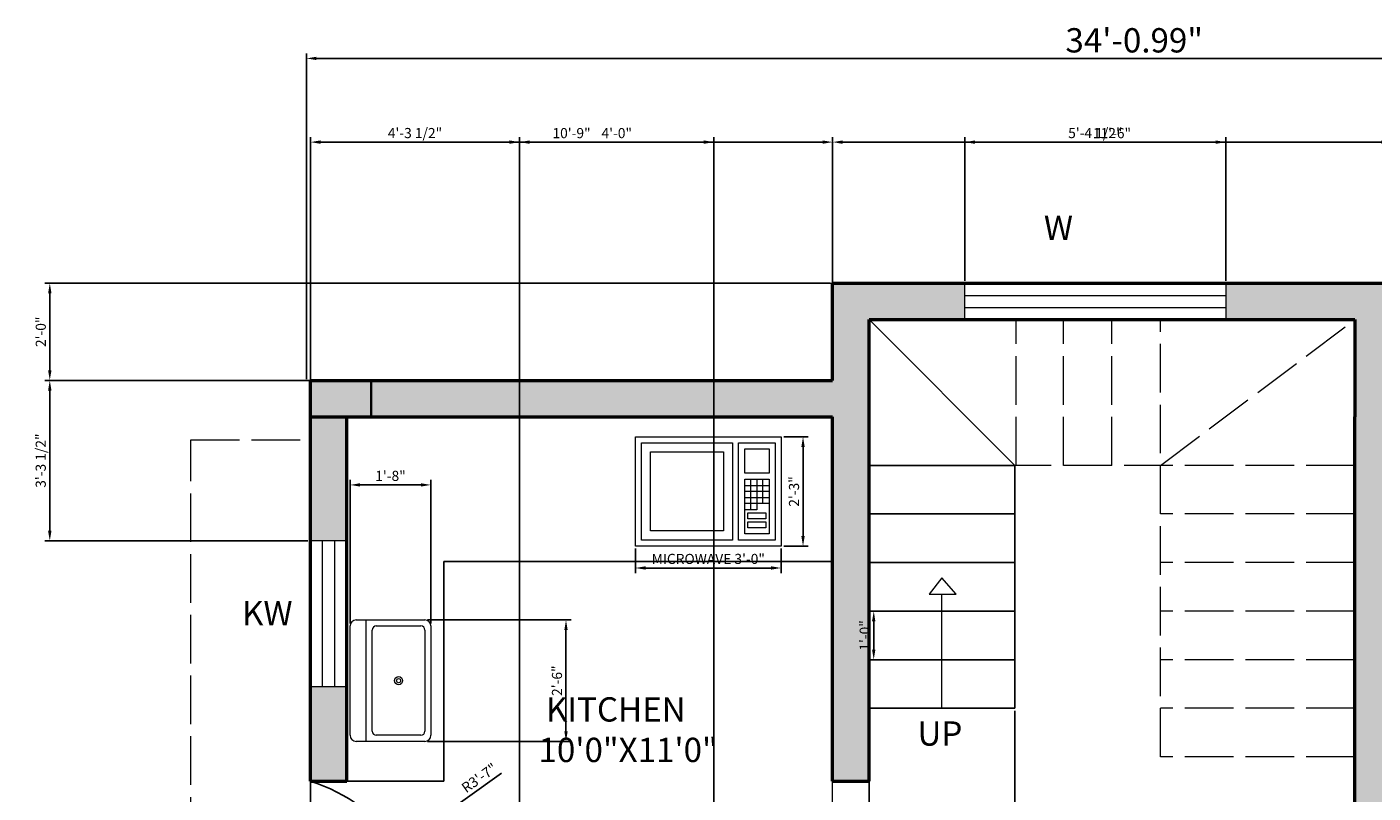
# Model space of a CAD drawing. Units: inches. Extents: x 5703 to 6226, y 10088 to 10813.
# Tile 4 of 5: x 5703 to 6036, y 10624 to 10813. Entities that reach past the tile are written whole.
import ezdxf

# ---------------------------------------------------------------- set-up
doc = ezdxf.new("R2010")
doc.units = ezdxf.units.IN
doc.linetypes.add('ACAD_ISO02W100', pattern=[15, 12, -3])
for name, color, linetype, lineweight in [('A-ANNO-DIMS', 2, 'Continuous', 18), ('A-ANNO-SYMB', 7, 'Continuous', 18), ('A-ANNO-TEXT', 7, 'Continuous', 18), ('A-AREA-IDEN', 7, 'Continuous', 18), ('A-COLS', 7, 'Continuous', 35), ('A-COLS-PATT', 7, 'Continuous', 13), ('A-DOOR', 140, 'Continuous', 25), ('A-EQPM', 8, 'Continuous', 18), ('A-FLOR-CASE', 8, 'Continuous', 25), ('A-FLOR-FIXT', 8, 'Continuous', 18), ('A-FLOR-STRS', 7, 'Continuous', 25), ('A-WALL', 7, 'Continuous', 50), ('A-WALL-PATT', 9, 'Continuous', 13)]:
    doc.layers.add(name, color=color, linetype=linetype, lineweight=lineweight)
for name, color, linetype, lineweight, true_color in [('A-FLOR-STRS-OVHD', 217, 'ACAD_ISO02W100', 18, 0x93278f), ('A-GLAZ', 112, 'Continuous', 18, 0x1ce368), ('A-ROOF-OVHD', 30, 'ACAD_ISO02W100', 18, 0xf8991e), ('A-WALL-OVHD', 30, 'ACAD_ISO02W100', 18, 0xf8991e)]:
    doc.layers.add(name, color=color, linetype=linetype, lineweight=lineweight, true_color=true_color)
doc.styles.get("Standard").update_dxf_attribs({"font": 'arial.ttf'})
doc.dimstyles.new('ISO-25', dxfattribs={"dimtxt": 2.5, "dimasz": 2.5, "dimexe": 1.25, "dimexo": 0.625, "dimtad": 1, "dimlunit": 3, "dimtxsty": 'Standard', "dimcen": 2.5, "dimadec": 0, "dimazin": 0, "dimtfac": 1, "dimtmove": 0, "dimatfit": 3, "dimfxl": 1, "dimarcsym": 0})

# ---------------------------------------------------------------- blocks, each defined once
blk = doc.blocks.new('*D10')
at = {"layer": 'A-ANNO-DIMS', "color": 0, "lineweight": -2, "transparency": 16777216}
for p, q in [((5772.18, 10726.21), (5772.18, 10806.65)), ((5774.68, 10805.4), (6178.68, 10805.4)), ((6181.18, 10726.49), (6181.18, 10806.65))]:
    blk.add_line(p, q, dxfattribs=at)
at = {"layer": 'A-ANNO-DIMS', "color": 0, "transparency": 16777216}
for points in [[(5774.68, 10805.81), (5774.68, 10804.98), (5772.18, 10805.4)], [(6178.68, 10805.81), (6178.68, 10804.98), (6181.18, 10805.4)]]:
    blk.add_solid(points, dxfattribs=at)
at = {"layer": 'Defpoints', "color": 0, "transparency": 16777216}
for p in [(6181.18, 10805.4), (5772.18, 10725.59), (6181.18, 10725.87)]:
    blk.add_point(p, dxfattribs=at)
at = {"layer": 'A-ANNO-DIMS', "color": 0, "transparency": 16777216, "insert": (5976.68, 10809.09), "char_height": 6, "attachment_point": 5}
blk.add_mtext('34\'-0.99"', dxfattribs=at)
blk = doc.blocks.new('Microwave')
for p, q in [((18, 10), (22, 10)), ((22, 9), (18, 9)), ((19, 7), (19, 11)), ((20, 11), (20, 7)), ((21, 7), (21, 11)), ((18, 8), (22, 8)), ((22, 7), (18, 7)), ((19, 6), (19, 7)), ((20, 7), (20, 6)), ((20, 6), (18, 6))]:
    blk.add_line(p, q)
for points in [[(0, 0), (0, 18), (24, 18), (24, 0)], [(1, 1), (1, 17), (16, 17), (16, 1)], [(17, 1), (17, 17), (23, 17), (23, 1)], [(18, 12), (18, 16), (22, 16), (22, 12)], [(2.5, 2.5), (2.5, 15.5), (14.5, 15.5), (14.5, 2.5)], [(18, 2), (18, 11), (22, 11), (22, 2)], [(18.5, 4.5), (18.5, 5.5), (21.5, 5.5), (21.5, 4.5)], [(18.5, 3), (18.5, 4), (21.5, 4), (21.5, 3)]]:
    blk.add_lwpolyline(points, close=True)
blk = doc.blocks.new('Sink-single - 30 in top')
blk.add_line((-15, -3.999996), (15, -3.999996))
for points in [[(-13.5, 0), (13.5, 0)], [(-15, -18.499996), (-15, -1.5)], [(15, -1.5), (15, -18.499996)], [(-13.5, -17.499996), (-13.5, -6.499996)], [(-12.5, -5.499996), (12.5, -5.499996)], [(13.5, -6.499996), (13.5, -17.499996)], [(12.5, -18.499996), (-12.5, -18.499996)], [(13.5, -19.999996), (-13.5, -19.999996)]]:
    blk.add_lwpolyline(points)
for radius in [1, 0.5]:
    blk.add_circle((0, -11.999996), radius)
for centre, radius, start, end in [((-13.5, -1.5), 1.5, 90, 180), ((13.5, -1.5), 1.5, 0, 90), ((-12.5, -6.499996), 1, 90, 180), ((12.5, -6.499996), 1, 0, 90), ((-13.5, -18.499996), 1.5, 180, 270), ((-12.5, -17.499996), 1, 180, 270), ((12.5, -17.499996), 1, 270, 0), ((13.5, -18.499996), 1.5, 270, 0)]:
    blk.add_arc(centre, radius, start, end)
blk = doc.blocks.new('WIN-36x9')
for p, q in [((0, 9), (0, 0)), ((36, 9), (0, 9)), ((36, 0), (36, 9)), ((36, 6), (0, 6)), ((36, 3), (0, 3)), ((0, 0), (36, 0))]:
    blk.add_line(p, q)
blk = doc.blocks.new('*D28')
at = {"layer": 'A-ANNO-DIMS', "color": 0, "lineweight": -2, "transparency": 16777216}
for p, q in [((5853.46, 10684.31), (5853.46, 10678.28)), ((5889.46, 10684.31), (5889.46, 10678.28)), ((5855.96, 10679.53), (5886.96, 10679.53))]:
    blk.add_line(p, q, dxfattribs=at)
at = {"layer": 'A-ANNO-DIMS', "color": 0, "transparency": 16777216}
for points in [[(5855.96, 10679.95), (5855.96, 10679.12), (5853.46, 10679.53)], [(5886.96, 10679.95), (5886.96, 10679.12), (5889.46, 10679.53)]]:
    blk.add_solid(points, dxfattribs=at)
at = {"layer": 'Defpoints', "color": 0, "transparency": 16777216}
for p in [(5853.46, 10684.93), (5889.46, 10684.93), (5889.46, 10679.53)]:
    blk.add_point(p, dxfattribs=at)
at = {"layer": 'A-ANNO-DIMS', "color": 0, "transparency": 16777216, "insert": (5871.46, 10681.45), "char_height": 2.5, "attachment_point": 5}
blk.add_mtext('MICROWAVE 3\'-0"', dxfattribs=at)
blk = doc.blocks.new('*D29')
at = {"layer": 'A-ANNO-DIMS', "color": 0, "lineweight": -2, "transparency": 16777216}
for p, q in [((5890.09, 10711.93), (5896.11, 10711.93)), ((5894.86, 10687.43), (5894.86, 10709.43)), ((5890.09, 10684.93), (5896.11, 10684.93))]:
    blk.add_line(p, q, dxfattribs=at)
at = {"layer": 'A-ANNO-DIMS', "color": 0, "transparency": 16777216}
for points in [[(5894.45, 10709.43), (5895.28, 10709.43), (5894.86, 10711.93)], [(5894.45, 10687.43), (5895.28, 10687.43), (5894.86, 10684.93)]]:
    blk.add_solid(points, dxfattribs=at)
at = {"layer": 'Defpoints', "color": 0, "transparency": 16777216}
for p in [(5889.46, 10711.93), (5894.86, 10711.93), (5889.46, 10684.93)]:
    blk.add_point(p, dxfattribs=at)
at = {"layer": 'A-ANNO-DIMS', "color": 0, "transparency": 16777216, "insert": (5892.96, 10698.43), "char_height": 2.5, "attachment_point": 5, "rotation": 90}
blk.add_mtext('2\'-3"', dxfattribs=at)
blk = doc.blocks.new('*D36')
at = {"layer": 'A-ANNO-DIMS', "color": 0, "lineweight": -2, "transparency": 16777216}
for p, q in [((5782.96, 10665.83), (5782.96, 10701.3)), ((5802.96, 10665.83), (5802.96, 10701.3)), ((5785.46, 10700.05), (5800.46, 10700.05))]:
    blk.add_line(p, q, dxfattribs=at)
at = {"layer": 'A-ANNO-DIMS', "color": 0, "transparency": 16777216}
for points in [[(5785.46, 10700.47), (5785.46, 10699.64), (5782.96, 10700.05)], [(5800.46, 10700.47), (5800.46, 10699.64), (5802.96, 10700.05)]]:
    blk.add_solid(points, dxfattribs=at)
at = {"layer": 'Defpoints', "color": 0, "transparency": 16777216}
for p in [(5802.96, 10700.05), (5782.96, 10665.2), (5802.96, 10665.2)]:
    blk.add_point(p, dxfattribs=at)
at = {"layer": 'A-ANNO-DIMS', "color": 0, "transparency": 16777216, "insert": (5792.96, 10701.96), "char_height": 2.5, "attachment_point": 5}
blk.add_mtext('1\'-8"', dxfattribs=at)
blk = doc.blocks.new('*D37')
at = {"layer": 'A-ANNO-DIMS', "color": 0, "lineweight": -2, "transparency": 16777216}
for p, q in [((5802.09, 10666.7), (5837.56, 10666.7)), ((5836.31, 10664.2), (5836.31, 10639.2)), ((5802.09, 10636.7), (5837.56, 10636.7))]:
    blk.add_line(p, q, dxfattribs=at)
at = {"layer": 'A-ANNO-DIMS', "color": 0, "transparency": 16777216}
for points in [[(5835.9, 10664.2), (5836.73, 10664.2), (5836.31, 10666.7)], [(5835.9, 10639.2), (5836.73, 10639.2), (5836.31, 10636.7)]]:
    blk.add_solid(points, dxfattribs=at)
at = {"layer": 'Defpoints', "color": 0, "transparency": 16777216}
for p in [(5801.46, 10666.7), (5801.46, 10636.7), (5836.31, 10636.7)]:
    blk.add_point(p, dxfattribs=at)
at = {"layer": 'A-ANNO-DIMS', "color": 0, "transparency": 16777216, "insert": (5834.41, 10651.7), "char_height": 2.5, "attachment_point": 5, "rotation": 90}
blk.add_mtext('2\'-6"', dxfattribs=at)
blk = doc.blocks.new('*D40')
at = {"layer": 'A-ANNO-DIMS', "color": 0, "lineweight": -2, "transparency": 16777216}
for p, q in [((5911.18, 10644.24), (5911.18, 10088.29)), ((5947.18, 10644.24), (5947.18, 10088.29)), ((5913.68, 10089.54), (5944.68, 10089.54))]:
    blk.add_line(p, q, dxfattribs=at)
at = {"layer": 'A-ANNO-DIMS', "color": 0, "transparency": 16777216}
for points in [[(5913.68, 10089.96), (5913.68, 10089.12), (5911.18, 10089.54)], [(5944.68, 10089.96), (5944.68, 10089.12), (5947.18, 10089.54)]]:
    blk.add_solid(points, dxfattribs=at)
at = {"layer": 'Defpoints', "color": 0, "transparency": 16777216}
for p in [(5911.18, 10644.87), (5947.18, 10644.87), (5947.18, 10089.54)]:
    blk.add_point(p, dxfattribs=at)
at = {"layer": 'A-ANNO-DIMS', "color": 0, "transparency": 16777216, "insert": (5929.18, 10091.44), "char_height": 2.5, "attachment_point": 5}
blk.add_mtext('3\'-0"', dxfattribs=at)
blk = doc.blocks.new('*D41')
at = {"layer": 'A-ANNO-DIMS', "color": 0, "lineweight": -2, "transparency": 16777216}
for p, q in [((5946.55, 10668.87), (5911.08, 10668.87)), ((5912.33, 10659.37), (5912.33, 10666.37)), ((5946.55, 10656.87), (5911.08, 10656.87))]:
    blk.add_line(p, q, dxfattribs=at)
at = {"layer": 'A-ANNO-DIMS', "color": 0, "transparency": 16777216}
for points in [[(5911.91, 10666.37), (5912.74, 10666.37), (5912.33, 10668.87)], [(5911.91, 10659.37), (5912.74, 10659.37), (5912.33, 10656.87)]]:
    blk.add_solid(points, dxfattribs=at)
at = {"layer": 'Defpoints', "color": 0, "transparency": 16777216}
for p in [(5912.33, 10668.87), (5947.18, 10668.87), (5947.18, 10656.87)]:
    blk.add_point(p, dxfattribs=at)
at = {"layer": 'A-ANNO-DIMS', "color": 0, "transparency": 16777216, "insert": (5910.42, 10662.87), "char_height": 2.5, "attachment_point": 5, "rotation": 90}
blk.add_mtext('1\'-0"', dxfattribs=at)
blk = doc.blocks.new('*D43')
at = {"layer": 'A-ANNO-DIMS', "color": 0, "lineweight": -2, "transparency": 16777216}
for p, q in [((5773.18, 10726.49), (5773.18, 10785.97)), ((5775.68, 10784.72), (5899.68, 10784.72)), ((5902.18, 10726.49), (5902.18, 10785.97))]:
    blk.add_line(p, q, dxfattribs=at)
at = {"layer": 'A-ANNO-DIMS', "color": 0, "transparency": 16777216}
for points in [[(5775.68, 10785.14), (5775.68, 10784.3), (5773.18, 10784.72)], [(5899.68, 10785.14), (5899.68, 10784.3), (5902.18, 10784.72)]]:
    blk.add_solid(points, dxfattribs=at)
at = {"layer": 'Defpoints', "color": 0, "transparency": 16777216}
for p in [(5902.18, 10784.72), (5773.18, 10725.87), (5902.18, 10725.87)]:
    blk.add_point(p, dxfattribs=at)
at = {"layer": 'A-ANNO-DIMS', "color": 0, "transparency": 16777216, "insert": (5837.68, 10786.62), "char_height": 2.5, "attachment_point": 5}
blk.add_mtext('10\'-9"', dxfattribs=at)
blk = doc.blocks.new('*D44')
at = {"layer": 'A-ANNO-DIMS', "color": 0, "lineweight": -2, "transparency": 16777216}
for p, q in [((5902.18, 10750.49), (5902.18, 10785.97)), ((5904.68, 10784.72), (6037.68, 10784.72)), ((6040.18, 10750.49), (6040.18, 10785.97))]:
    blk.add_line(p, q, dxfattribs=at)
at = {"layer": 'A-ANNO-DIMS', "color": 0, "transparency": 16777216}
for points in [[(5904.68, 10785.14), (5904.68, 10784.3), (5902.18, 10784.72)], [(6037.68, 10785.14), (6037.68, 10784.3), (6040.18, 10784.72)]]:
    blk.add_solid(points, dxfattribs=at)
at = {"layer": 'Defpoints', "color": 0, "transparency": 16777216}
for p in [(6040.18, 10784.72), (5902.18, 10749.87), (6040.18, 10749.87)]:
    blk.add_point(p, dxfattribs=at)
at = {"layer": 'A-ANNO-DIMS', "color": 0, "transparency": 16777216, "insert": (5971.18, 10786.62), "char_height": 2.5, "attachment_point": 5}
blk.add_mtext('11\'-6"', dxfattribs=at)
blk = doc.blocks.new('*D45')
at = {"layer": 'A-ANNO-DIMS', "color": 0, "lineweight": -2, "transparency": 16777216}
for p, q in [((5901.55, 10749.87), (5707.55, 10749.87)), ((5708.8, 10728.37), (5708.8, 10747.37)), ((5901.55, 10725.87), (5707.55, 10725.87))]:
    blk.add_line(p, q, dxfattribs=at)
at = {"layer": 'A-ANNO-DIMS', "color": 0, "transparency": 16777216}
for points in [[(5708.38, 10747.37), (5709.22, 10747.37), (5708.8, 10749.87)], [(5708.38, 10728.37), (5709.22, 10728.37), (5708.8, 10725.87)]]:
    blk.add_solid(points, dxfattribs=at)
at = {"layer": 'Defpoints', "color": 0, "transparency": 16777216}
for p in [(5708.8, 10749.87), (5902.18, 10749.87), (5902.18, 10725.87)]:
    blk.add_point(p, dxfattribs=at)
at = {"layer": 'A-ANNO-DIMS', "color": 0, "transparency": 16777216, "insert": (5706.9, 10737.87), "char_height": 2.5, "attachment_point": 5, "rotation": 90}
blk.add_mtext('2\'-0"', dxfattribs=at)
blk = doc.blocks.new('*D46')
at = {"layer": 'A-ANNO-DIMS', "color": 0, "lineweight": -2, "transparency": 16777216}
for p, q in [((5934.86, 10750.49), (5934.86, 10785.97)), ((5937.36, 10784.72), (5996.77, 10784.72)), ((5999.27, 10750.49), (5999.27, 10785.97))]:
    blk.add_line(p, q, dxfattribs=at)
at = {"layer": 'A-ANNO-DIMS', "color": 0, "transparency": 16777216}
for points in [[(5937.36, 10785.14), (5937.36, 10784.3), (5934.86, 10784.72)], [(5996.77, 10785.14), (5996.77, 10784.3), (5999.27, 10784.72)]]:
    blk.add_solid(points, dxfattribs=at)
at = {"layer": 'Defpoints', "color": 0, "transparency": 16777216}
for p in [(5999.27, 10784.72), (5934.86, 10749.87), (5999.27, 10749.87)]:
    blk.add_point(p, dxfattribs=at)
at = {"layer": 'A-ANNO-DIMS', "color": 0, "transparency": 16777216, "insert": (5967.07, 10786.64), "char_height": 2.5, "attachment_point": 5}
blk.add_mtext('5\'-4 1/2"', dxfattribs=at)
blk = doc.blocks.new('*D47')
at = {"layer": 'A-ANNO-DIMS', "color": 0, "lineweight": -2, "transparency": 16777216}
for p, q in [((5824.85, 10313.99), (5824.85, 10785.97)), ((5827.35, 10784.72), (5870.35, 10784.72)), ((5872.85, 10313.99), (5872.85, 10785.97))]:
    blk.add_line(p, q, dxfattribs=at)
at = {"layer": 'A-ANNO-DIMS', "color": 0, "transparency": 16777216}
for points in [[(5827.35, 10785.14), (5827.35, 10784.3), (5824.85, 10784.72)], [(5870.35, 10785.14), (5870.35, 10784.3), (5872.85, 10784.72)]]:
    blk.add_solid(points, dxfattribs=at)
at = {"layer": 'Defpoints', "color": 0, "transparency": 16777216}
for p in [(5872.85, 10784.72), (5824.85, 10313.37), (5872.85, 10313.37)]:
    blk.add_point(p, dxfattribs=at)
at = {"layer": 'A-ANNO-DIMS', "color": 0, "transparency": 16777216, "insert": (5848.85, 10786.62), "char_height": 2.5, "attachment_point": 5}
blk.add_mtext('4\'-0"', dxfattribs=at)
blk = doc.blocks.new('*D48')
at = {"layer": 'A-ANNO-DIMS', "color": 0, "lineweight": -2, "transparency": 16777216}
for p, q in [((5773.18, 10304.99), (5773.18, 10785.97)), ((5775.68, 10784.72), (5822.35, 10784.72)), ((5824.85, 10304.99), (5824.85, 10785.97))]:
    blk.add_line(p, q, dxfattribs=at)
at = {"layer": 'A-ANNO-DIMS', "color": 0, "transparency": 16777216}
for points in [[(5775.68, 10785.14), (5775.68, 10784.3), (5773.18, 10784.72)], [(5822.35, 10785.14), (5822.35, 10784.3), (5824.85, 10784.72)]]:
    blk.add_solid(points, dxfattribs=at)
at = {"layer": 'Defpoints', "color": 0, "transparency": 16777216}
for p in [(5824.85, 10784.72), (5773.18, 10304.37), (5824.85, 10304.37)]:
    blk.add_point(p, dxfattribs=at)
at = {"layer": 'A-ANNO-DIMS', "color": 0, "transparency": 16777216, "insert": (5799.01, 10786.64), "char_height": 2.5, "attachment_point": 5}
blk.add_mtext('4\'-3 1/2"', dxfattribs=at)
blk = doc.blocks.new('*D50')
at = {"layer": 'A-ANNO-DIMS', "color": 0, "lineweight": -2, "transparency": 16777216}
for p, q in [((5772.55, 10725.87), (5707.55, 10725.87)), ((5708.8, 10688.73), (5708.8, 10723.37)), ((5772.55, 10686.23), (5707.55, 10686.23))]:
    blk.add_line(p, q, dxfattribs=at)
at = {"layer": 'A-ANNO-DIMS', "color": 0, "transparency": 16777216}
for points in [[(5708.38, 10723.37), (5709.22, 10723.37), (5708.8, 10725.87)], [(5708.38, 10688.73), (5709.22, 10688.73), (5708.8, 10686.23)]]:
    blk.add_solid(points, dxfattribs=at)
at = {"layer": 'Defpoints', "color": 0, "transparency": 16777216}
for p in [(5708.8, 10725.87), (5773.18, 10725.87), (5773.18, 10686.23)]:
    blk.add_point(p, dxfattribs=at)
at = {"layer": 'A-ANNO-DIMS', "color": 0, "transparency": 16777216, "insert": (5706.88, 10706.05), "char_height": 2.5, "attachment_point": 5, "rotation": 90}
blk.add_mtext('3\'-3 1/2"', dxfattribs=at)
blk = doc.blocks.new('*D58')
at = {"layer": 'A-ANNO-DIMS', "color": 0, "lineweight": -2, "transparency": 16777216}
for p, q in [((5820.36, 10628.86), (5797.21, 10612.32)), ((5760.18, 10585.87), (5795.18, 10610.87))]:
    blk.add_line(p, q, dxfattribs=at)
at = {"layer": 'A-ANNO-DIMS', "color": 0, "transparency": 16777216}
blk.add_solid([(5796.97, 10612.66), (5797.45, 10611.98), (5795.18, 10610.87)], dxfattribs=at)
at = {"layer": 'Defpoints', "color": 0, "transparency": 16777216}
for p in [(5795.18, 10610.87), (5760.18, 10585.87)]:
    blk.add_point(p, dxfattribs=at)
at = {"layer": 'A-ANNO-DIMS', "color": 0, "transparency": 16777216, "insert": (5815.07, 10627.42), "char_height": 2.5, "attachment_point": 5, "rotation": 35.5383}
blk.add_mtext('R3\'-7"', dxfattribs=at)

msp = doc.modelspace()

# ---------------------------------------------------------------- hatches: boundary and pattern name
at = {"layer": 'A-COLS-PATT'}
h = msp.add_hatch(color=256, dxfattribs=at)
h.dxf.hatch_style = 1
h.paths.add_polyline_path([(5788.176, 10725.869), (5773.176, 10725.869), (5773.176, 10716.869), (5788.176, 10716.869)])
h.paths.add_polyline_path([(5782.176, 10516.684), (5773.176, 10516.684), (5773.176, 10497.849), (5782.176, 10497.849)])
h.paths.add_polyline_path([(5782.176, 10319.369), (5773.176, 10319.369), (5773.176, 10304.369), (5782.176, 10304.369)])
h.paths.add_polyline_path([(5960.955, 10313.369), (5953.525, 10313.369), (5953.525, 10304.369), (5960.955, 10304.369)])
h.paths.add_polyline_path([(6040.176, 10314.869), (6031.176, 10314.869), (6031.176, 10304.369), (6040.176, 10304.369)])
h.paths.add_polyline_path([(6181.176, 10198.545), (6172.176, 10198.545), (6172.176, 10178.369), (6181.176, 10178.369)])
h.paths.add_polyline_path([(6181.176, 10505.369), (6172.176, 10505.369), (6172.176, 10492.633), (6181.176, 10492.633)])
h.paths.add_polyline_path([(6181.176, 10725.869), (6166.176, 10725.869), (6166.176, 10716.869), (6181.176, 10716.869)])
at = {"layer": 'A-WALL-PATT'}
h = msp.add_hatch(color=256, dxfattribs=at)
h.dxf.hatch_style = 1
h.paths.add_polyline_path([(6057.982, 10725.869), (6040.176, 10725.869), (6040.176, 10749.869), (5999.271, 10749.869), (5999.271, 10740.869), (6031.176, 10740.869), (6031.176, 10716.869), (6031.176, 10511.369), (6013.525, 10511.369), (6013.525, 10505.369), (6048.161, 10505.369), (6048.161, 10511.369), (6040.176, 10511.369), (6040.176, 10716.869), (6057.982, 10716.869)])
h.paths.add_polyline_path([(6166.176, 10725.869), (6093.982, 10725.869), (6093.982, 10716.869), (6166.176, 10716.869)])
h.paths.add_polyline_path([(6181.176, 10716.869), (6172.176, 10716.869), (6172.176, 10511.369), (6132.161, 10511.369, -0.0172363), (6132.161, 10509.369), (6132.161, 10505.369), (6181.176, 10505.369)])
h.paths.add_polyline_path([(6181.176, 10468.633), (6172.176, 10468.633), (6172.176, 10451.369), (6098.676, 10451.369), (6098.676, 10505.369), (6102.161, 10505.369), (6102.161, 10511.369), (6090.161, 10511.369), (6090.161, 10507.369, -0.0121933), (6090.161, 10505.369), (6092.676, 10505.369), (6092.676, 10451.369), (6085.668, 10451.369), (6085.668, 10445.369), (6092.676, 10445.369), (6172.176, 10445.369), (6172.176, 10342.529), (6181.176, 10342.529)])
h.paths.add_polyline_path([(6181.176, 10282.529), (6172.176, 10282.529), (6172.176, 10253.369), (6092.676, 10253.369), (6092.676, 10247.369), (6094.176, 10247.369), (6094.176, 10238.954), (6100.176, 10238.954), (6100.176, 10247.369), (6172.176, 10247.369), (6172.176, 10234.545), (6181.176, 10234.545)])
h.paths.add_polyline_path([(6172.176, 10187.369), (6100.176, 10187.369), (6100.176, 10220.954), (6096.176, 10220.954, -0.0293864), (6094.176, 10220.954), (6094.176, 10178.369), (6172.176, 10178.369)])
h.paths.add_polyline_path([(6050.745, 10187.369), (6040.176, 10187.369), (6040.176, 10178.369), (6050.745, 10178.369)])
h.paths.add_polyline_path([(6040.176, 10187.369), (6031.176, 10187.369), (6031.176, 10178.369), (6040.176, 10178.369)])
h.paths.add_polyline_path([(6040.176, 10304.369), (6031.176, 10304.369), (6031.176, 10187.369), (6040.176, 10187.369)])
h.paths.add_polyline_path([(6040.176, 10393.328), (6031.176, 10393.328), (6031.176, 10314.869), (6040.176, 10314.869)])
h.paths.add_polyline_path([(6040.176, 10445.369), (6046.458, 10445.369), (6046.458, 10451.369), (6031.176, 10451.369), (6031.176, 10408.328), (6040.176, 10408.328)])
h.paths.add_polyline_path([(5911.176, 10584.869), (5845.666, 10584.869, -0.0172363), (5845.666, 10582.869), (5845.666, 10578.869), (5902.176, 10578.869), (5902.176, 10505.369), (5953.525, 10505.369), (5953.525, 10511.369), (5911.176, 10511.369)])
h.paths.add_polyline_path([(5902.176, 10511.369), (5782.176, 10511.369), (5782.176, 10505.369), (5902.176, 10505.369)])
h.paths.add_polyline_path([(5782.176, 10578.869), (5815.666, 10578.869), (5815.666, 10584.869), (5773.176, 10584.869), (5773.176, 10516.684), (5782.176, 10516.684)])
h.paths.add_polyline_path([(5782.176, 10497.849), (5773.176, 10497.849), (5773.176, 10438.429), (5782.176, 10438.429)])
h.paths.add_polyline_path([(5782.176, 10378.429), (5773.176, 10378.429), (5773.176, 10319.369), (5782.176, 10319.369)])
h.paths.add_polyline_path([(5824.846, 10313.369), (5782.176, 10313.369), (5782.176, 10304.369), (5824.846, 10304.369)])
h.paths.add_polyline_path([(5953.525, 10313.369), (5872.846, 10313.369), (5872.846, 10304.369), (5953.525, 10304.369)])
h = msp.add_hatch(color=256, dxfattribs=at)
h.dxf.hatch_style = 1
h.paths.add_polyline_path([(5911.176, 10740.869), (5934.861, 10740.869), (5934.861, 10749.869), (5902.176, 10749.869), (5902.176, 10725.869), (5788.176, 10725.869), (5788.176, 10716.869), (5902.176, 10716.869), (5902.176, 10626.869), (5911.176, 10626.869), (5911.176, 10716.869)])
h = msp.add_hatch(color=256, dxfattribs=at)
h.dxf.hatch_style = 1
h.paths.add_polyline_path([(5782.176, 10650.231), (5773.176, 10650.231), (5773.176, 10626.869), (5782.176, 10626.869)])
h.paths.add_polyline_path([(5782.176, 10716.869), (5773.176, 10716.869), (5773.176, 10686.231), (5782.176, 10686.231)])

# ---------------------------------------------------------------- linework, layer by layer
at = {"layer": 'A-ANNO-SYMB'}
for p, q in [((5929.176, 10677.088), (5926.052, 10673.027)), ((5932.678, 10673.027), (5929.176, 10677.088)), ((5926.052, 10673.027), (5929.176, 10673.027)), ((5929.176, 10644.869), (5929.176, 10673.027)), ((5929.176, 10673.027), (5932.678, 10673.027))]:
    msp.add_line(p, q, dxfattribs=at)
at = {"layer": 'A-COLS'}
for p, q in [((5788.176, 10716.869), (5788.176, 10725.869)), ((5773.176, 10716.869), (5788.176, 10716.869))]:
    msp.add_line(p, q, dxfattribs=at)
at = {"layer": 'A-DOOR'}
msp.add_arc((5760.176, 10585.869), 43.012, 358.66778, 72.40758, dxfattribs=at)
at = {"layer": 'A-FLOR-CASE'}
for p, q in [((5806.176, 10626.869), (5806.176, 10681.103)), ((5806.176, 10681.103), (5902.176, 10681.103)), ((5782.176, 10626.869), (5806.176, 10626.869))]:
    msp.add_line(p, q, dxfattribs=at)
at = {"layer": 'A-FLOR-STRS'}
for p, q in [((5947.176, 10704.869), (5911.176, 10740.869)), ((5911.176, 10704.869), (5947.176, 10704.869)), ((5947.176, 10644.869), (5947.176, 10704.869)), ((5911.176, 10692.869), (5947.176, 10692.869)), ((5911.176, 10680.869), (5947.176, 10680.869)), ((5911.176, 10668.869), (5947.176, 10668.869)), ((5911.176, 10656.869), (5947.176, 10656.869)), ((5911.176, 10644.869), (5947.176, 10644.869))]:
    msp.add_line(p, q, dxfattribs=at)
at = {"layer": 'A-FLOR-STRS-OVHD'}
for p, q in [((5947.528, 10704.869), (5947.528, 10740.869)), ((5959.176, 10704.869), (5959.176, 10740.869)), ((5971.176, 10704.869), (5971.176, 10740.869)), ((5983.176, 10704.869), (6031.176, 10740.869)), ((5983.176, 10632.869), (5983.176, 10740.869)), ((6031.176, 10704.869), (5947.176, 10704.869)), ((6031.176, 10692.869), (5983.176, 10692.869)), ((6031.176, 10680.869), (5983.176, 10680.869)), ((6031.176, 10668.869), (5983.176, 10668.869)), ((6031.176, 10656.869), (5983.176, 10656.869)), ((6031.176, 10644.869), (5983.176, 10644.869)), ((6031.176, 10632.869), (5983.176, 10632.869))]:
    msp.add_line(p, q, dxfattribs=at)
at = {"layer": 'A-GLAZ'}
for p, q in [((5934.861, 10740.869), (5934.861, 10749.869)), ((5934.861, 10749.869), (5971.176, 10749.869)), ((5971.176, 10749.869), (5971.176, 10749.869)), ((5971.176, 10749.869), (5999.271, 10749.869)), ((5999.271, 10749.869), (5999.271, 10740.869)), ((5934.861, 10746.869), (5971.176, 10746.869)), ((5934.861, 10743.869), (5971.176, 10743.869)), ((5971.176, 10746.869), (5999.271, 10746.869)), ((5971.176, 10743.869), (5999.271, 10743.869)), ((5934.861, 10740.869), (5999.271, 10740.869))]:
    msp.add_line(p, q, dxfattribs=at)
at = {"layer": 'A-ROOF-OVHD'}
for p, q in [((5773.176, 10725.869), (5773.176, 10749.869)), ((5773.176, 10749.869), (5902.176, 10749.869)), ((5743.649, 10565.956), (5743.649, 10711.167)), ((5743.649, 10711.167), (5773.176, 10711.167))]:
    msp.add_line(p, q, dxfattribs=at)
at = {"layer": 'A-WALL'}
for p, q in [((5902.176, 10725.869), (5902.176, 10749.869)), ((5902.176, 10749.869), (6040.176, 10749.869)), ((5911.176, 10716.869), (5911.176, 10740.869)), ((5911.176, 10740.869), (6031.176, 10740.869)), ((6031.176, 10740.869), (6031.176, 10716.869)), ((5773.176, 10725.869), (5902.176, 10725.869)), ((5773.176, 10626.869), (5773.176, 10725.869)), ((5773.176, 10716.869), (5902.176, 10716.869)), ((5782.176, 10626.869), (5782.176, 10716.869)), ((5902.176, 10626.869), (5902.176, 10716.869)), ((5911.176, 10626.869), (5911.176, 10716.869)), ((6031.176, 10511.369), (6031.176, 10716.869)), ((5773.176, 10626.869), (5782.176, 10626.869)), ((5902.176, 10626.869), (5911.176, 10626.869))]:
    msp.add_line(p, q, dxfattribs=at)
at = {"layer": 'A-WALL-OVHD'}
for p, q in [((5902.176, 10584.869), (5902.176, 10626.869)), ((5911.176, 10584.869), (5911.176, 10626.869))]:
    msp.add_line(p, q, dxfattribs=at)

# ---------------------------------------------------------------- block references
at = {"layer": 'A-EQPM', "xscale": 1.5, "yscale": 1.5, "zscale": 1.5}
msp.add_blockref('Microwave', (5853.463, 10684.933), dxfattribs=at)
at = {"layer": 'A-FLOR-FIXT', "rotation": 90}
msp.add_blockref('Sink-single - 30 in top', (5782.962, 10651.705), dxfattribs=at)
at = {"layer": 'A-GLAZ', "rotation": 270.0000000000116}
msp.add_blockref('WIN-36x9', (5773.177, 10686.231), dxfattribs=at)

# ---------------------------------------------------------------- texts
at = {"layer": 'A-ANNO-TEXT', "char_height": 6, "attachment_point": 1}
for s, insert in [(' W', (5952.527, 10766.566)), (' KW', (5754.455, 10671.354)), ('    UP', (5915.799, 10641.659))]:
    msp.add_mtext_dynamic_manual_height_columns(s, width=71.13425, gutter_width=12.5, heights=[0], dxfattribs=dict(at, insert=insert))
at = {"layer": 'A-AREA-IDEN', "insert": (5829.528, 10647.601), "char_height": 6, "attachment_point": 1}
msp.add_mtext_dynamic_manual_height_columns(' KITCHEN\\P10\'0"X11\'0"', width=71.13425, gutter_width=12.5, heights=[0], dxfattribs=at)

# ---------------------------------------------------------------- dimensions: what is measured, and where the dimension line sits
at = {"layer": 'A-ANNO-DIMS'}
for base, p1, p2, override, picture, middle in [((6181.176, 10805.396), (5772.182, 10725.59), (6181.176, 10725.869), {"dimtxt": 6, "dimclrd": 0, "dimclre": 0, "dimclrt": 0}, '*D10', (5976.679, 10809.086)), ((5824.846, 10784.719), (5773.176, 10304.369), (5824.846, 10304.369), {"dimdec": 1, "dimlfac": 1, "dimrnd": 0, "dimzin": 1, "dimdsep": 46, "dimlunit": 4, "dimfrac": 2}, '*D48', (5799.011, 10786.637)), ((5902.176, 10784.719), (5773.176, 10725.869), (5902.176, 10725.869), {"dimdec": 1, "dimlfac": 1, "dimrnd": 0, "dimzin": 1, "dimdsep": 46, "dimlunit": 4, "dimfrac": 2}, '*D43', (5837.676, 10786.62)), ((5872.846, 10784.719), (5824.846, 10313.369), (5872.846, 10313.369), {"dimdec": 1, "dimlfac": 1, "dimrnd": 0, "dimzin": 1, "dimdsep": 46, "dimlunit": 4, "dimfrac": 2}, '*D47', (5848.846, 10786.62)), ((6040.176, 10784.719), (5902.176, 10749.869), (6040.176, 10749.869), {"dimdec": 1, "dimlfac": 1, "dimrnd": 0, "dimzin": 1, "dimdsep": 46, "dimlunit": 4, "dimfrac": 2}, '*D44', (5971.176, 10786.62)), ((5999.271, 10784.719), (5934.861, 10749.869), (5999.271, 10749.869), {"dimdec": 1, "dimlfac": 1, "dimrnd": 0, "dimzin": 1, "dimdsep": 46, "dimlunit": 4, "dimfrac": 2}, '*D46', (5967.066, 10786.636)), ((5802.962, 10700.055), (5782.962, 10665.205), (5802.962, 10665.205), {"dimdec": 1, "dimlfac": 1, "dimrnd": 0, "dimzin": 1, "dimdsep": 46, "dimlunit": 4, "dimfrac": 2}, '*D36', (5792.962, 10701.956)), ((5947.176, 10089.539), (5911.176, 10644.869), (5947.176, 10644.869), {"dimdec": 1, "dimlfac": 1, "dimrnd": 0, "dimzin": 1, "dimdsep": 46, "dimlunit": 4, "dimfrac": 2}, '*D40', (5929.176, 10091.442))]:
    dim = msp.add_linear_dim(base=base, p1=p1, p2=p2, dimstyle='ISO-25', override=override, dxfattribs=at)
    dim.commit()
    dim.dimension.update_dxf_attribs({"geometry": picture, "text_midpoint": middle})
for base, p1, p2, angle, picture, middle in [((5708.799, 10749.869), (5902.176, 10725.869), (5902.176, 10749.869), 90, '*D45', (5706.897, 10737.869)), ((5708.799, 10725.869), (5773.176, 10686.231), (5773.176, 10725.869), 90, '*D50', (5706.88, 10706.05)), ((5894.863, 10711.933), (5889.463, 10684.933), (5889.463, 10711.933), 90, '*D29', (5892.961, 10698.433)), ((5912.326, 10668.869), (5947.176, 10656.869), (5947.176, 10668.869), 90, '*D41', (5910.425, 10662.869)), ((5836.312, 10636.705), (5801.462, 10666.705), (5801.462, 10636.705), 270, '*D37', (5834.41, 10651.705))]:
    dim = msp.add_linear_dim(base=base, p1=p1, p2=p2, angle=angle, dimstyle='ISO-25', override={"dimdec": 1, "dimlfac": 1, "dimrnd": 0, "dimzin": 1, "dimdsep": 46, "dimlunit": 4, "dimfrac": 2}, dxfattribs=at)
    dim.commit()
    dim.dimension.update_dxf_attribs({"geometry": picture, "text_midpoint": middle})
dim = msp.add_linear_dim(base=(5889.463, 10679.533), p1=(5853.463, 10684.933), p2=(5889.463, 10684.933), text='MICROWAVE <>', dimstyle='ISO-25', override={"dimdec": 1, "dimlfac": 1, "dimrnd": 0, "dimzin": 1, "dimdsep": 46, "dimlunit": 4, "dimfrac": 2}, dxfattribs=at)
dim.commit()
dim.dimension.update_dxf_attribs({"geometry": '*D28', "text_midpoint": (5871.463, 10681.452)})
dim = msp.add_radius_dim(center=(5760.176, 10585.869), mpoint=(5795.176, 10610.869), dimstyle='ISO-25', override={"dimdec": 1, "dimlfac": 1, "dimrnd": 0, "dimzin": 1, "dimdsep": 46, "dimlunit": 4, "dimfrac": 2}, dxfattribs=at)
dim.commit()
dim.dimension.update_dxf_attribs({"geometry": '*D58', "text_midpoint": (5816.176, 10625.869), "dimtype": 164})

doc.saveas('drawing.dxf')
